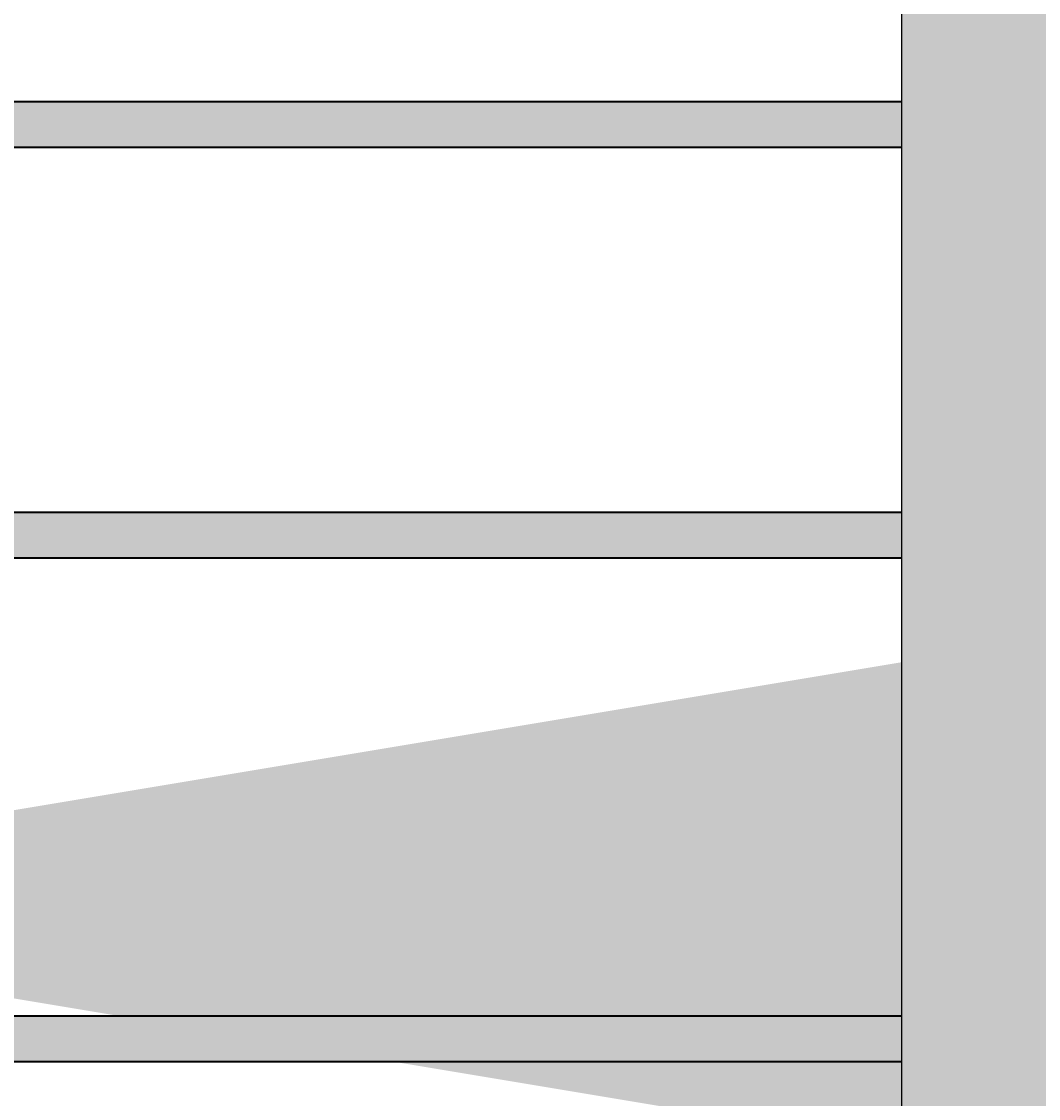
# Model space of a CAD drawing. Units: millimetres. Extents: x -22994 to 29398, y -19990 to 20176.
# Tile 20 of 135: x 77 to 99, y 76 to 99. Entities that reach past the tile are written whole.
import ezdxf

# ---------------------------------------------------------------- set-up
doc = ezdxf.new("R2010")
doc.units = ezdxf.units.MM
doc.header["$MEASUREMENT"] = 0
for name, color, linetype, lineweight in [('M-DIMS', 2, 'Continuous', 18), ('M-EQPM', 7, 'Continuous', 25), ('M-EQPM-PATT', 7, 'Continuous', 18), ('M-PIPE', 7, 'Continuous', 35)]:
    doc.layers.add(name, color=color, linetype=linetype, lineweight=lineweight)
doc.styles.get("Standard").update_dxf_attribs({"font": 'arial.ttf'})
doc.dimstyles.get("Standard").update_dxf_attribs({"dimtxt": 0.18, "dimasz": 10000, "dimexe": 0.18, "dimexo": 0.0625, "dimgap": 0.09, "dimtad": 0, "dimtih": 1, "dimtoh": 1, "dimdec": 0, "dimzin": 0, "dimdsep": 46, "dimtxsty": 'Standard', "dimcen": 0.09, "dimadec": 0, "dimazin": 0, "dimtfac": 1, "dimtdec": 0, "dimtofl": 0, "dimtmove": 0, "dimatfit": 3, "dimfxl": 1, "dimtolj": 1, "dimtzin": 0, "dimlwd": 30, "dimarcsym": 0})

# ---------------------------------------------------------------- blocks, each defined once
blk = doc.blocks.new('*D2')
at = {"layer": 'Defpoints', "color": 0, "transparency": 16777216}
for p in [(6.677, 10.271), (290.852, 10.271), (290.852, -5.079)]:
    blk.add_point(p, dxfattribs=at)
at = {"layer": 'M-DIMS', "color": 0, "lineweight": -2, "transparency": 16777216}
for p, q in [((6.677, 10.209), (6.677, -5.259)), ((290.852, 10.209), (290.852, -5.259))]:
    blk.add_line(p, q, dxfattribs=at)
at = {"layer": 'M-DIMS', "color": 0, "lineweight": 30, "transparency": 16777216}
for p, q in [((-9993.323, -5.079), (-19993.323, -5.079)), ((10290.852, -5.079), (20290.852, -5.079))]:
    blk.add_line(p, q, dxfattribs=at)
at = {"layer": 'M-DIMS', "color": 0, "transparency": 16777216}
for points in [[(-9993.323, 1661.588), (-9993.323, -1671.745), (6.677, -5.079)], [(10290.852, 1661.588), (10290.852, -1671.745), (290.852, -5.079)]]:
    blk.add_solid(points, dxfattribs=at)
at = {"layer": 'M-DIMS', "color": 0, "transparency": 16777216, "insert": (148.765, -5.079), "char_height": 0.18, "attachment_point": 5}
blk.add_mtext('\\A1;284.2', dxfattribs=at)
blk = doc.blocks.new('*D3')
at = {"layer": 'Defpoints', "color": 0, "transparency": 16777216}
for p in [(110.265, 204.165), (110.265, 176.366), (95.833, 127.967)]:
    blk.add_point(p, dxfattribs=at)
at = {"layer": 'M-DIMS', "color": 0, "lineweight": -2, "transparency": 16777216}
for p, q in [((95.833, 128.03), (95.833, 204.345)), ((110.265, 176.429), (110.265, 204.345))]:
    blk.add_line(p, q, dxfattribs=at)
at = {"layer": 'M-DIMS', "color": 0, "lineweight": 30, "transparency": 16777216}
for p, q in [((-9904.167, 204.165), (-19904.167, 204.165)), ((10110.265, 204.165), (20110.265, 204.165))]:
    blk.add_line(p, q, dxfattribs=at)
at = {"layer": 'M-DIMS', "color": 0, "transparency": 16777216}
for points in [[(-9904.167, 1870.832), (-9904.167, -1462.501), (95.833, 204.165)], [(10110.265, 1870.832), (10110.265, -1462.501), (110.265, 204.165)]]:
    blk.add_solid(points, dxfattribs=at)
at = {"layer": 'M-DIMS', "color": 0, "transparency": 16777216, "insert": (103.049, 204.165), "char_height": 0.18, "attachment_point": 5}
blk.add_mtext('\\A1;14.432', dxfattribs=at)
blk = doc.blocks.new('*D4')
at = {"layer": 'Defpoints', "color": 0, "transparency": 16777216}
for p in [(116.265, 204.165), (110.265, 176.366), (116.265, 176.366)]:
    blk.add_point(p, dxfattribs=at)
at = {"layer": 'M-DIMS', "color": 0, "lineweight": -2, "transparency": 16777216}
for p, q in [((110.265, 176.429), (110.265, 204.345)), ((116.265, 176.429), (116.265, 204.345))]:
    blk.add_line(p, q, dxfattribs=at)
at = {"layer": 'M-DIMS', "color": 0, "lineweight": 30, "transparency": 16777216}
for p, q in [((-9889.735, 204.165), (-19889.735, 204.165)), ((10116.265, 204.165), (20116.265, 204.165))]:
    blk.add_line(p, q, dxfattribs=at)
at = {"layer": 'M-DIMS', "color": 0, "transparency": 16777216}
for points in [[(-9889.735, 1870.832), (-9889.735, -1462.501), (110.265, 204.165)], [(10116.265, 1870.832), (10116.265, -1462.501), (116.265, 204.165)]]:
    blk.add_solid(points, dxfattribs=at)
at = {"layer": 'M-DIMS', "color": 0, "transparency": 16777216, "insert": (113.265, 204.165), "char_height": 0.18, "attachment_point": 5}
blk.add_mtext('\\A1;6', dxfattribs=at)
blk = doc.blocks.new('*D5')
at = {"layer": 'Defpoints', "color": 0, "transparency": 16777216}
for p in [(181.265, 204.165), (116.265, 176.366), (181.265, 176.366)]:
    blk.add_point(p, dxfattribs=at)
at = {"layer": 'M-DIMS', "color": 0, "lineweight": -2, "transparency": 16777216}
for p, q in [((116.265, 176.429), (116.265, 204.345)), ((181.265, 176.429), (181.265, 204.345))]:
    blk.add_line(p, q, dxfattribs=at)
at = {"layer": 'M-DIMS', "color": 0, "lineweight": 30, "transparency": 16777216}
for p, q in [((-9883.735, 204.165), (-19883.735, 204.165)), ((10181.265, 204.165), (20181.265, 204.165))]:
    blk.add_line(p, q, dxfattribs=at)
at = {"layer": 'M-DIMS', "color": 0, "transparency": 16777216}
for points in [[(-9883.735, 1870.832), (-9883.735, -1462.501), (116.265, 204.165)], [(10181.265, 1870.832), (10181.265, -1462.501), (181.265, 204.165)]]:
    blk.add_solid(points, dxfattribs=at)
at = {"layer": 'M-DIMS', "color": 0, "transparency": 16777216, "insert": (148.765, 204.165), "char_height": 0.18, "attachment_point": 5}
blk.add_mtext('\\A1;65', dxfattribs=at)
blk = doc.blocks.new('*D6')
at = {"layer": 'Defpoints', "color": 0, "transparency": 16777216}
for p in [(187.265, 204.165), (181.265, 176.366), (187.265, 176.366)]:
    blk.add_point(p, dxfattribs=at)
at = {"layer": 'M-DIMS', "color": 0, "lineweight": -2, "transparency": 16777216}
for p, q in [((181.265, 176.429), (181.265, 204.345)), ((187.265, 176.429), (187.265, 204.345))]:
    blk.add_line(p, q, dxfattribs=at)
at = {"layer": 'M-DIMS', "color": 0, "lineweight": 30, "transparency": 16777216}
for p, q in [((-9818.735, 204.165), (-19818.735, 204.165)), ((10187.265, 204.165), (20187.265, 204.165))]:
    blk.add_line(p, q, dxfattribs=at)
at = {"layer": 'M-DIMS', "color": 0, "transparency": 16777216}
for points in [[(-9818.735, 1870.832), (-9818.735, -1462.501), (181.265, 204.165)], [(10187.265, 1870.832), (10187.265, -1462.501), (187.265, 204.165)]]:
    blk.add_solid(points, dxfattribs=at)
at = {"layer": 'M-DIMS', "color": 0, "transparency": 16777216, "insert": (184.265, 204.165), "char_height": 0.18, "attachment_point": 5}
blk.add_mtext('\\A1;6', dxfattribs=at)
blk = doc.blocks.new('*D7')
at = {"layer": 'Defpoints', "color": 0, "transparency": 16777216}
for p in [(201.697, 204.165), (187.265, 176.366), (201.697, 127.967)]:
    blk.add_point(p, dxfattribs=at)
at = {"layer": 'M-DIMS', "color": 0, "lineweight": -2, "transparency": 16777216}
for p, q in [((187.265, 176.429), (187.265, 204.345)), ((201.697, 128.03), (201.697, 204.345))]:
    blk.add_line(p, q, dxfattribs=at)
at = {"layer": 'M-DIMS', "color": 0, "lineweight": 30, "transparency": 16777216}
for p, q in [((-9812.735, 204.165), (-19812.735, 204.165)), ((10201.697, 204.165), (20201.697, 204.165))]:
    blk.add_line(p, q, dxfattribs=at)
at = {"layer": 'M-DIMS', "color": 0, "transparency": 16777216}
for points in [[(-9812.735, 1870.832), (-9812.735, -1462.501), (187.265, 204.165)], [(10201.697, 1870.832), (10201.697, -1462.501), (201.697, 204.165)]]:
    blk.add_solid(points, dxfattribs=at)
at = {"layer": 'M-DIMS', "color": 0, "transparency": 16777216, "insert": (194.481, 204.165), "char_height": 0.18, "attachment_point": 5}
blk.add_mtext('\\A1;14.432', dxfattribs=at)
blk = doc.blocks.new('*D8')
at = {"layer": 'Defpoints', "color": 0, "transparency": 16777216}
for p in [(227.648, 204.165), (227.648, 146.73), (201.697, 127.967)]:
    blk.add_point(p, dxfattribs=at)
at = {"layer": 'M-DIMS', "color": 0, "lineweight": -2, "transparency": 16777216}
for p, q in [((201.697, 128.03), (201.697, 204.345)), ((227.648, 146.792), (227.648, 204.345))]:
    blk.add_line(p, q, dxfattribs=at)
at = {"layer": 'M-DIMS', "color": 0, "lineweight": 30, "transparency": 16777216}
for p, q in [((-9798.303, 204.165), (-19798.303, 204.165)), ((10227.648, 204.165), (20227.648, 204.165))]:
    blk.add_line(p, q, dxfattribs=at)
at = {"layer": 'M-DIMS', "color": 0, "transparency": 16777216}
for points in [[(-9798.303, 1870.832), (-9798.303, -1462.501), (201.697, 204.165)], [(10227.648, 1870.832), (10227.648, -1462.501), (227.648, 204.165)]]:
    blk.add_solid(points, dxfattribs=at)
at = {"layer": 'M-DIMS', "color": 0, "transparency": 16777216, "insert": (214.673, 204.165), "char_height": 0.18, "attachment_point": 5}
blk.add_mtext('\\A1;25.95', dxfattribs=at)
blk = doc.blocks.new('*D9')
at = {"layer": 'Defpoints', "color": 0, "transparency": 16777216}
for p in [(187.265, 176.366), (306.202, 176.366), (290.852, 10.271)]:
    blk.add_point(p, dxfattribs=at)
at = {"layer": 'M-DIMS', "color": 0, "lineweight": 30, "transparency": 16777216}
for p, q in [((306.202, 10176.366), (306.202, 20176.366)), ((306.202, -9989.729), (306.202, -19989.729))]:
    blk.add_line(p, q, dxfattribs=at)
at = {"layer": 'M-DIMS', "color": 0, "lineweight": -2, "transparency": 16777216}
for p, q in [((187.327, 176.366), (306.382, 176.366)), ((290.915, 10.271), (306.382, 10.271))]:
    blk.add_line(p, q, dxfattribs=at)
at = {"layer": 'M-DIMS', "color": 0, "transparency": 16777216}
for points in [[(-1360.465, 10176.366), (1972.869, 10176.366), (306.202, 176.366)], [(-1360.465, -9989.729), (1972.869, -9989.729), (306.202, 10.271)]]:
    blk.add_solid(points, dxfattribs=at)
at = {"layer": 'M-DIMS', "color": 0, "transparency": 16777216, "insert": (306.202, 93.319), "char_height": 0.18, "attachment_point": 5}
blk.add_mtext('\\A1;166.1', dxfattribs=at)
blk = doc.blocks.new('*D10')
at = {"layer": 'Defpoints', "color": 0, "transparency": 16777216}
for p in [(125.65, 136.071), (133.346, 136.071), (133.346, -5.079)]:
    blk.add_point(p, dxfattribs=at)
at = {"layer": 'M-DIMS', "color": 0, "lineweight": -2, "transparency": 16777216}
for p, q in [((125.65, 136.009), (125.65, -5.259)), ((133.346, 136.009), (133.346, -5.259))]:
    blk.add_line(p, q, dxfattribs=at)
at = {"layer": 'M-DIMS', "color": 0, "lineweight": 30, "transparency": 16777216}
for p, q in [((-9874.35, -5.079), (-19874.35, -5.079)), ((10133.346, -5.079), (20133.346, -5.079))]:
    blk.add_line(p, q, dxfattribs=at)
at = {"layer": 'M-DIMS', "color": 0, "transparency": 16777216}
for points in [[(-9874.35, 1661.588), (-9874.35, -1671.745), (125.65, -5.079)], [(10133.346, 1661.588), (10133.346, -1671.745), (133.346, -5.079)]]:
    blk.add_solid(points, dxfattribs=at)
at = {"layer": 'M-DIMS', "color": 0, "transparency": 16777216, "insert": (129.498, -5.079), "char_height": 0.18, "attachment_point": 5}
blk.add_mtext('\\A1;7.696', dxfattribs=at)
blk = doc.blocks.new('*D11')
at = {"layer": 'Defpoints', "color": 0, "transparency": 16777216}
for p in [(133.346, 136.071), (135.65, 136.071), (135.65, -5.079)]:
    blk.add_point(p, dxfattribs=at)
at = {"layer": 'M-DIMS', "color": 0, "lineweight": -2, "transparency": 16777216}
for p, q in [((133.346, 136.009), (133.346, -5.259)), ((135.65, 136.009), (135.65, -5.259))]:
    blk.add_line(p, q, dxfattribs=at)
at = {"layer": 'M-DIMS', "color": 0, "lineweight": 30, "transparency": 16777216}
for p, q in [((-9866.654, -5.079), (-19866.654, -5.079)), ((10135.65, -5.079), (20135.65, -5.079))]:
    blk.add_line(p, q, dxfattribs=at)
at = {"layer": 'M-DIMS', "color": 0, "transparency": 16777216}
for points in [[(-9866.654, 1661.588), (-9866.654, -1671.745), (133.346, -5.079)], [(10135.65, 1661.588), (10135.65, -1671.745), (135.65, -5.079)]]:
    blk.add_solid(points, dxfattribs=at)
at = {"layer": 'M-DIMS', "color": 0, "transparency": 16777216, "insert": (134.498, -5.079), "char_height": 0.18, "attachment_point": 5}
blk.add_mtext('\\A1;2.304', dxfattribs=at)
blk = doc.blocks.new('*D12')
at = {"layer": 'Defpoints', "color": 0, "transparency": 16777216}
for p in [(135.65, 136.071), (145.65, 136.071), (145.65, -5.079)]:
    blk.add_point(p, dxfattribs=at)
at = {"layer": 'M-DIMS', "color": 0, "lineweight": -2, "transparency": 16777216}
for p, q in [((135.65, 136.009), (135.65, -5.259)), ((145.65, 136.009), (145.65, -5.259))]:
    blk.add_line(p, q, dxfattribs=at)
at = {"layer": 'M-DIMS', "color": 0, "lineweight": 30, "transparency": 16777216}
for p, q in [((-9864.35, -5.079), (-19864.35, -5.079)), ((10145.65, -5.079), (20145.65, -5.079))]:
    blk.add_line(p, q, dxfattribs=at)
at = {"layer": 'M-DIMS', "color": 0, "transparency": 16777216}
for points in [[(-9864.35, 1661.588), (-9864.35, -1671.745), (135.65, -5.079)], [(10145.65, 1661.588), (10145.65, -1671.745), (145.65, -5.079)]]:
    blk.add_solid(points, dxfattribs=at)
at = {"layer": 'M-DIMS', "color": 0, "transparency": 16777216, "insert": (140.65, -5.079), "char_height": 0.18, "attachment_point": 5}
blk.add_mtext('\\A1;10', dxfattribs=at)
blk = doc.blocks.new('*D13')
at = {"layer": 'Defpoints', "color": 0, "transparency": 16777216}
for p in [(145.65, 136.071), (155.65, 136.071), (155.65, -5.079)]:
    blk.add_point(p, dxfattribs=at)
at = {"layer": 'M-DIMS', "color": 0, "lineweight": -2, "transparency": 16777216}
for p, q in [((145.65, 136.009), (145.65, -5.259)), ((155.65, 136.009), (155.65, -5.259))]:
    blk.add_line(p, q, dxfattribs=at)
at = {"layer": 'M-DIMS', "color": 0, "lineweight": 30, "transparency": 16777216}
for p, q in [((-9854.35, -5.079), (-19854.35, -5.079)), ((10155.65, -5.079), (20155.65, -5.079))]:
    blk.add_line(p, q, dxfattribs=at)
at = {"layer": 'M-DIMS', "color": 0, "transparency": 16777216}
for points in [[(-9854.35, 1661.588), (-9854.35, -1671.745), (145.65, -5.079)], [(10155.65, 1661.588), (10155.65, -1671.745), (155.65, -5.079)]]:
    blk.add_solid(points, dxfattribs=at)
at = {"layer": 'M-DIMS', "color": 0, "transparency": 16777216, "insert": (150.65, -5.079), "char_height": 0.18, "attachment_point": 5}
blk.add_mtext('\\A1;10', dxfattribs=at)
blk = doc.blocks.new('*D14')
at = {"layer": 'Defpoints', "color": 0, "transparency": 16777216}
for p in [(155.65, 136.071), (165.65, 136.071), (165.65, -5.079)]:
    blk.add_point(p, dxfattribs=at)
at = {"layer": 'M-DIMS', "color": 0, "lineweight": -2, "transparency": 16777216}
for p, q in [((155.65, 136.009), (155.65, -5.259)), ((165.65, 136.009), (165.65, -5.259))]:
    blk.add_line(p, q, dxfattribs=at)
at = {"layer": 'M-DIMS', "color": 0, "lineweight": 30, "transparency": 16777216}
for p, q in [((-9844.35, -5.079), (-19844.35, -5.079)), ((10165.65, -5.079), (20165.65, -5.079))]:
    blk.add_line(p, q, dxfattribs=at)
at = {"layer": 'M-DIMS', "color": 0, "transparency": 16777216}
for points in [[(-9844.35, 1661.588), (-9844.35, -1671.745), (155.65, -5.079)], [(10165.65, 1661.588), (10165.65, -1671.745), (165.65, -5.079)]]:
    blk.add_solid(points, dxfattribs=at)
at = {"layer": 'M-DIMS', "color": 0, "transparency": 16777216, "insert": (160.65, -5.079), "char_height": 0.18, "attachment_point": 5}
blk.add_mtext('\\A1;10', dxfattribs=at)
blk = doc.blocks.new('*D15')
at = {"layer": 'Defpoints', "color": 0, "transparency": 16777216}
for p in [(173.346, 154.788), (173.346, 136.071), (306.202, 136.071)]:
    blk.add_point(p, dxfattribs=at)
at = {"layer": 'M-DIMS', "color": 0, "lineweight": 30, "transparency": 16777216}
for p, q in [((306.202, 10154.788), (306.202, 20154.788)), ((306.202, -9863.929), (306.202, -19863.929))]:
    blk.add_line(p, q, dxfattribs=at)
at = {"layer": 'M-DIMS', "color": 0, "lineweight": -2, "transparency": 16777216}
for p, q in [((173.408, 154.788), (306.382, 154.788)), ((173.408, 136.071), (306.382, 136.071))]:
    blk.add_line(p, q, dxfattribs=at)
at = {"layer": 'M-DIMS', "color": 0, "transparency": 16777216}
for points in [[(-1360.465, 10154.788), (1972.869, 10154.788), (306.202, 154.788)], [(-1360.465, -9863.929), (1972.869, -9863.929), (306.202, 136.071)]]:
    blk.add_solid(points, dxfattribs=at)
at = {"layer": 'M-DIMS', "color": 0, "transparency": 16777216, "insert": (306.202, 145.43), "char_height": 0.18, "attachment_point": 5}
blk.add_mtext('\\A1;18.717', dxfattribs=at)
blk = doc.blocks.new('*D16')
at = {"layer": 'Defpoints', "color": 0, "transparency": 16777216}
for p in [(120.17, 204.165), (110.466, 48.035), (120.17, 48.035)]:
    blk.add_point(p, dxfattribs=at)
at = {"layer": 'M-DIMS', "color": 0, "lineweight": -2, "transparency": 16777216}
for p, q in [((110.466, 48.097), (110.466, 204.345)), ((120.17, 48.097), (120.17, 204.345))]:
    blk.add_line(p, q, dxfattribs=at)
at = {"layer": 'M-DIMS', "color": 0, "lineweight": 30, "transparency": 16777216}
for p, q in [((-9889.534, 204.165), (-19889.534, 204.165)), ((10120.17, 204.165), (20120.17, 204.165))]:
    blk.add_line(p, q, dxfattribs=at)
at = {"layer": 'M-DIMS', "color": 0, "transparency": 16777216}
for points in [[(-9889.534, 1870.832), (-9889.534, -1462.501), (110.466, 204.165)], [(10120.17, 1870.832), (10120.17, -1462.501), (120.17, 204.165)]]:
    blk.add_solid(points, dxfattribs=at)
at = {"layer": 'M-DIMS', "color": 0, "transparency": 16777216, "insert": (115.318, 204.165), "char_height": 0.18, "attachment_point": 5}
blk.add_mtext('\\A1;9.704', dxfattribs=at)
blk = doc.blocks.new('*D17')
at = {"layer": 'Defpoints', "color": 0, "transparency": 16777216}
for p in [(126.17, 204.165), (120.17, 48.035), (126.17, 48.035)]:
    blk.add_point(p, dxfattribs=at)
at = {"layer": 'M-DIMS', "color": 0, "lineweight": -2, "transparency": 16777216}
for p, q in [((120.17, 48.097), (120.17, 204.345)), ((126.17, 48.097), (126.17, 204.345))]:
    blk.add_line(p, q, dxfattribs=at)
at = {"layer": 'M-DIMS', "color": 0, "lineweight": 30, "transparency": 16777216}
for p, q in [((-9879.83, 204.165), (-19879.83, 204.165)), ((10126.17, 204.165), (20126.17, 204.165))]:
    blk.add_line(p, q, dxfattribs=at)
at = {"layer": 'M-DIMS', "color": 0, "transparency": 16777216}
for points in [[(-9879.83, 1870.832), (-9879.83, -1462.501), (120.17, 204.165)], [(10126.17, 1870.832), (10126.17, -1462.501), (126.17, 204.165)]]:
    blk.add_solid(points, dxfattribs=at)
at = {"layer": 'M-DIMS', "color": 0, "transparency": 16777216, "insert": (123.17, 204.165), "char_height": 0.18, "attachment_point": 5}
blk.add_mtext('\\A1;6', dxfattribs=at)
blk = doc.blocks.new('*D18')
at = {"layer": 'Defpoints', "color": 0, "transparency": 16777216}
for p in [(132.17, 204.165), (126.17, 48.035), (132.17, 48.035)]:
    blk.add_point(p, dxfattribs=at)
at = {"layer": 'M-DIMS', "color": 0, "lineweight": -2, "transparency": 16777216}
for p, q in [((126.17, 48.097), (126.17, 204.345)), ((132.17, 48.097), (132.17, 204.345))]:
    blk.add_line(p, q, dxfattribs=at)
at = {"layer": 'M-DIMS', "color": 0, "lineweight": 30, "transparency": 16777216}
for p, q in [((-9873.83, 204.165), (-19873.83, 204.165)), ((10132.17, 204.165), (20132.17, 204.165))]:
    blk.add_line(p, q, dxfattribs=at)
at = {"layer": 'M-DIMS', "color": 0, "transparency": 16777216}
for points in [[(-9873.83, 1870.832), (-9873.83, -1462.501), (126.17, 204.165)], [(10132.17, 1870.832), (10132.17, -1462.501), (132.17, 204.165)]]:
    blk.add_solid(points, dxfattribs=at)
at = {"layer": 'M-DIMS', "color": 0, "transparency": 16777216, "insert": (129.17, 204.165), "char_height": 0.18, "attachment_point": 5}
blk.add_mtext('\\A1;6', dxfattribs=at)
blk = doc.blocks.new('*D19')
at = {"layer": 'Defpoints', "color": 0, "transparency": 16777216}
for p in [(138.17, 204.165), (132.17, 48.035), (138.17, 48.035)]:
    blk.add_point(p, dxfattribs=at)
at = {"layer": 'M-DIMS', "color": 0, "lineweight": -2, "transparency": 16777216}
for p, q in [((132.17, 48.097), (132.17, 204.345)), ((138.17, 48.097), (138.17, 204.345))]:
    blk.add_line(p, q, dxfattribs=at)
at = {"layer": 'M-DIMS', "color": 0, "lineweight": 30, "transparency": 16777216}
for p, q in [((-9867.83, 204.165), (-19867.83, 204.165)), ((10138.17, 204.165), (20138.17, 204.165))]:
    blk.add_line(p, q, dxfattribs=at)
at = {"layer": 'M-DIMS', "color": 0, "transparency": 16777216}
for points in [[(-9867.83, 1870.832), (-9867.83, -1462.501), (132.17, 204.165)], [(10138.17, 1870.832), (10138.17, -1462.501), (138.17, 204.165)]]:
    blk.add_solid(points, dxfattribs=at)
at = {"layer": 'M-DIMS', "color": 0, "transparency": 16777216, "insert": (135.17, 204.165), "char_height": 0.18, "attachment_point": 5}
blk.add_mtext('\\A1;6', dxfattribs=at)
blk = doc.blocks.new('*D20')
at = {"layer": 'Defpoints', "color": 0, "transparency": 16777216}
for p in [(144.17, 204.165), (138.17, 48.035), (144.17, 48.035)]:
    blk.add_point(p, dxfattribs=at)
at = {"layer": 'M-DIMS', "color": 0, "lineweight": -2, "transparency": 16777216}
for p, q in [((138.17, 48.097), (138.17, 204.345)), ((144.17, 48.097), (144.17, 204.345))]:
    blk.add_line(p, q, dxfattribs=at)
at = {"layer": 'M-DIMS', "color": 0, "lineweight": 30, "transparency": 16777216}
for p, q in [((-9861.83, 204.165), (-19861.83, 204.165)), ((10144.17, 204.165), (20144.17, 204.165))]:
    blk.add_line(p, q, dxfattribs=at)
at = {"layer": 'M-DIMS', "color": 0, "transparency": 16777216}
for points in [[(-9861.83, 1870.832), (-9861.83, -1462.501), (138.17, 204.165)], [(10144.17, 1870.832), (10144.17, -1462.501), (144.17, 204.165)]]:
    blk.add_solid(points, dxfattribs=at)
at = {"layer": 'M-DIMS', "color": 0, "transparency": 16777216, "insert": (141.17, 204.165), "char_height": 0.18, "attachment_point": 5}
blk.add_mtext('\\A1;6', dxfattribs=at)
blk = doc.blocks.new('*D21')
at = {"layer": 'Defpoints', "color": 0, "transparency": 16777216}
for p in [(149.116, 204.165), (144.17, 48.035), (149.116, 48.035)]:
    blk.add_point(p, dxfattribs=at)
at = {"layer": 'M-DIMS', "color": 0, "lineweight": -2, "transparency": 16777216}
for p, q in [((144.17, 48.097), (144.17, 204.345)), ((149.116, 48.097), (149.116, 204.345))]:
    blk.add_line(p, q, dxfattribs=at)
at = {"layer": 'M-DIMS', "color": 0, "lineweight": 30, "transparency": 16777216}
for p, q in [((-9855.83, 204.165), (-19855.83, 204.165)), ((10149.116, 204.165), (20149.116, 204.165))]:
    blk.add_line(p, q, dxfattribs=at)
at = {"layer": 'M-DIMS', "color": 0, "transparency": 16777216}
for points in [[(-9855.83, 1870.832), (-9855.83, -1462.501), (144.17, 204.165)], [(10149.116, 1870.832), (10149.116, -1462.501), (149.116, 204.165)]]:
    blk.add_solid(points, dxfattribs=at)
at = {"layer": 'M-DIMS', "color": 0, "transparency": 16777216, "insert": (146.643, 204.165), "char_height": 0.18, "attachment_point": 5}
blk.add_mtext('\\A1;4.945', dxfattribs=at)
blk = doc.blocks.new('*D22')
at = {"layer": 'Defpoints', "color": 0, "transparency": 16777216}
for p in [(149.116, 30.99), (155.116, 30.99), (155.116, -5.079)]:
    blk.add_point(p, dxfattribs=at)
at = {"layer": 'M-DIMS', "color": 0, "lineweight": -2, "transparency": 16777216}
for p, q in [((149.116, 30.927), (149.116, -5.259)), ((155.116, 30.927), (155.116, -5.259))]:
    blk.add_line(p, q, dxfattribs=at)
at = {"layer": 'M-DIMS', "color": 0, "lineweight": 30, "transparency": 16777216}
for p, q in [((-9850.884, -5.079), (-19850.884, -5.079)), ((10155.116, -5.079), (20155.116, -5.079))]:
    blk.add_line(p, q, dxfattribs=at)
at = {"layer": 'M-DIMS', "color": 0, "transparency": 16777216}
for points in [[(-9850.884, 1661.588), (-9850.884, -1671.745), (149.116, -5.079)], [(10155.116, 1661.588), (10155.116, -1671.745), (155.116, -5.079)]]:
    blk.add_solid(points, dxfattribs=at)
at = {"layer": 'M-DIMS', "color": 0, "transparency": 16777216, "insert": (152.116, -5.079), "char_height": 0.18, "attachment_point": 5}
blk.add_mtext('\\A1;6', dxfattribs=at)
blk = doc.blocks.new('*D23')
at = {"layer": 'Defpoints', "color": 0, "transparency": 16777216}
for p in [(155.116, 30.99), (161.116, 30.99), (161.116, -5.079)]:
    blk.add_point(p, dxfattribs=at)
at = {"layer": 'M-DIMS', "color": 0, "lineweight": -2, "transparency": 16777216}
for p, q in [((155.116, 30.927), (155.116, -5.259)), ((161.116, 30.927), (161.116, -5.259))]:
    blk.add_line(p, q, dxfattribs=at)
at = {"layer": 'M-DIMS', "color": 0, "lineweight": 30, "transparency": 16777216}
for p, q in [((-9844.884, -5.079), (-19844.884, -5.079)), ((10161.116, -5.079), (20161.116, -5.079))]:
    blk.add_line(p, q, dxfattribs=at)
at = {"layer": 'M-DIMS', "color": 0, "transparency": 16777216}
for points in [[(-9844.884, 1661.588), (-9844.884, -1671.745), (155.116, -5.079)], [(10161.116, 1661.588), (10161.116, -1671.745), (161.116, -5.079)]]:
    blk.add_solid(points, dxfattribs=at)
at = {"layer": 'M-DIMS', "color": 0, "transparency": 16777216, "insert": (158.116, -5.079), "char_height": 0.18, "attachment_point": 5}
blk.add_mtext('\\A1;6', dxfattribs=at)
blk = doc.blocks.new('*D24')
at = {"layer": 'Defpoints', "color": 0, "transparency": 16777216}
for p in [(161.116, 30.99), (166.439, 30.99), (166.439, -5.079)]:
    blk.add_point(p, dxfattribs=at)
at = {"layer": 'M-DIMS', "color": 0, "lineweight": -2, "transparency": 16777216}
for p, q in [((161.116, 30.927), (161.116, -5.259)), ((166.439, 30.927), (166.439, -5.259))]:
    blk.add_line(p, q, dxfattribs=at)
at = {"layer": 'M-DIMS', "color": 0, "lineweight": 30, "transparency": 16777216}
for p, q in [((-9838.884, -5.079), (-19838.884, -5.079)), ((10166.439, -5.079), (20166.439, -5.079))]:
    blk.add_line(p, q, dxfattribs=at)
at = {"layer": 'M-DIMS', "color": 0, "transparency": 16777216}
for points in [[(-9838.884, 1661.588), (-9838.884, -1671.745), (161.116, -5.079)], [(10166.439, 1661.588), (10166.439, -1671.745), (166.439, -5.079)]]:
    blk.add_solid(points, dxfattribs=at)
at = {"layer": 'M-DIMS', "color": 0, "transparency": 16777216, "insert": (163.777, -5.079), "char_height": 0.18, "attachment_point": 5}
blk.add_mtext('\\A1;5.323', dxfattribs=at)
blk = doc.blocks.new('*D25')
at = {"layer": 'Defpoints', "color": 0, "transparency": 16777216}
for p in [(166.439, 30.99), (172.439, 30.99), (172.439, -5.079)]:
    blk.add_point(p, dxfattribs=at)
at = {"layer": 'M-DIMS', "color": 0, "lineweight": -2, "transparency": 16777216}
for p, q in [((166.439, 30.927), (166.439, -5.259)), ((172.439, 30.927), (172.439, -5.259))]:
    blk.add_line(p, q, dxfattribs=at)
at = {"layer": 'M-DIMS', "color": 0, "lineweight": 30, "transparency": 16777216}
for p, q in [((-9833.561, -5.079), (-19833.561, -5.079)), ((10172.439, -5.079), (20172.439, -5.079))]:
    blk.add_line(p, q, dxfattribs=at)
at = {"layer": 'M-DIMS', "color": 0, "transparency": 16777216}
for points in [[(-9833.561, 1661.588), (-9833.561, -1671.745), (166.439, -5.079)], [(10172.439, 1661.588), (10172.439, -1671.745), (172.439, -5.079)]]:
    blk.add_solid(points, dxfattribs=at)
at = {"layer": 'M-DIMS', "color": 0, "transparency": 16777216, "insert": (169.439, -5.079), "char_height": 0.18, "attachment_point": 5}
blk.add_mtext('\\A1;6', dxfattribs=at)
blk = doc.blocks.new('*D26')
at = {"layer": 'Defpoints', "color": 0, "transparency": 16777216}
for p in [(172.439, 30.99), (178.439, 30.99), (178.439, -5.079)]:
    blk.add_point(p, dxfattribs=at)
at = {"layer": 'M-DIMS', "color": 0, "lineweight": -2, "transparency": 16777216}
for p, q in [((172.439, 30.927), (172.439, -5.259)), ((178.439, 30.927), (178.439, -5.259))]:
    blk.add_line(p, q, dxfattribs=at)
at = {"layer": 'M-DIMS', "color": 0, "lineweight": 30, "transparency": 16777216}
for p, q in [((-9827.561, -5.079), (-19827.561, -5.079)), ((10178.439, -5.079), (20178.439, -5.079))]:
    blk.add_line(p, q, dxfattribs=at)
at = {"layer": 'M-DIMS', "color": 0, "transparency": 16777216}
for points in [[(-9827.561, 1661.588), (-9827.561, -1671.745), (172.439, -5.079)], [(10178.439, 1661.588), (10178.439, -1671.745), (178.439, -5.079)]]:
    blk.add_solid(points, dxfattribs=at)
at = {"layer": 'M-DIMS', "color": 0, "transparency": 16777216, "insert": (175.439, -5.079), "char_height": 0.18, "attachment_point": 5}
blk.add_mtext('\\A1;6', dxfattribs=at)
blk = doc.blocks.new('*D27')
at = {"layer": 'Defpoints', "color": 0, "transparency": 16777216}
for p in [(178.439, 30.99), (188.117, 30.99), (188.117, -5.079)]:
    blk.add_point(p, dxfattribs=at)
at = {"layer": 'M-DIMS', "color": 0, "lineweight": -2, "transparency": 16777216}
for p, q in [((178.439, 30.927), (178.439, -5.259)), ((188.117, 30.927), (188.117, -5.259))]:
    blk.add_line(p, q, dxfattribs=at)
at = {"layer": 'M-DIMS', "color": 0, "lineweight": 30, "transparency": 16777216}
for p, q in [((-9821.561, -5.079), (-19821.561, -5.079)), ((10188.117, -5.079), (20188.117, -5.079))]:
    blk.add_line(p, q, dxfattribs=at)
at = {"layer": 'M-DIMS', "color": 0, "transparency": 16777216}
for points in [[(-9821.561, 1661.588), (-9821.561, -1671.745), (178.439, -5.079)], [(10188.117, 1661.588), (10188.117, -1671.745), (188.117, -5.079)]]:
    blk.add_solid(points, dxfattribs=at)
at = {"layer": 'M-DIMS', "color": 0, "transparency": 16777216, "insert": (183.278, -5.079), "char_height": 0.18, "attachment_point": 5}
blk.add_mtext('\\A1;9.679', dxfattribs=at)
blk = doc.blocks.new('*D28')
at = {"layer": 'Defpoints', "color": 0, "transparency": 16777216}
for p in [(188.117, 48.035), (306.202, 48.035), (188.117, 30.99)]:
    blk.add_point(p, dxfattribs=at)
at = {"layer": 'M-DIMS', "color": 0, "lineweight": 30, "transparency": 16777216}
for p, q in [((306.202, 10048.035), (306.202, 20048.035)), ((306.202, -9969.01), (306.202, -19969.01))]:
    blk.add_line(p, q, dxfattribs=at)
at = {"layer": 'M-DIMS', "color": 0, "lineweight": -2, "transparency": 16777216}
for p, q in [((188.18, 48.035), (306.382, 48.035)), ((188.18, 30.99), (306.382, 30.99))]:
    blk.add_line(p, q, dxfattribs=at)
at = {"layer": 'M-DIMS', "color": 0, "transparency": 16777216}
for points in [[(-1360.465, 10048.035), (1972.869, 10048.035), (306.202, 48.035)], [(-1360.465, -9969.01), (1972.869, -9969.01), (306.202, 30.99)]]:
    blk.add_solid(points, dxfattribs=at)
at = {"layer": 'M-DIMS', "color": 0, "transparency": 16777216, "insert": (306.202, 39.512), "char_height": 0.18, "attachment_point": 5}
blk.add_mtext('\\A1;17.045', dxfattribs=at)
blk = doc.blocks.new('*D29')
at = {"layer": 'Defpoints', "color": 0, "transparency": 16777216}
for p in [(36.801, 80.045), (64.03, 80.045)]:
    blk.add_point(p, dxfattribs=at)
at = {"layer": 'M-DIMS', "color": 0, "lineweight": -2, "transparency": 16777216}
for p, q in [((50.325, 80.045), (50.505, 80.045)), ((50.415, 79.955), (50.415, 80.135))]:
    blk.add_line(p, q, dxfattribs=at)
at = {"layer": 'M-DIMS', "color": 0, "lineweight": 30, "transparency": 16777216}
blk.add_line((20064.03, 80.03), (10064.03, 80.038), dxfattribs=at)
at = {"layer": 'M-DIMS', "color": 0, "transparency": 16777216}
blk.add_solid([(10064.031, 1746.704), (10064.028, -1586.629), (64.03, 80.045)], dxfattribs=at)
at = {"layer": 'M-DIMS', "color": 0, "transparency": 16777216, "insert": (20064.521, 80.03), "char_height": 0.18, "attachment_point": 5}
blk.add_mtext('\\A1;∅27.23', dxfattribs=at)
blk = doc.blocks.new('*D36')
at = {"layer": 'Defpoints', "color": 0, "transparency": 16777216}
for p in [(46.39, 31.303), (46.387, 26.593)]:
    blk.add_point(p, dxfattribs=at)
at = {"layer": 'M-DIMS', "color": 0, "lineweight": 30, "transparency": 16777216}
for p, q in [((57.15, 20031.301), (51.77, 10031.302)), ((10057.15, 20031.301), (57.15, 20031.301))]:
    blk.add_line(p, q, dxfattribs=at)
at = {"layer": 'M-DIMS', "color": 0, "lineweight": -2, "transparency": 16777216}
for p, q in [((46.389, 28.858), (46.389, 29.038)), ((46.299, 28.948), (46.479, 28.948))]:
    blk.add_line(p, q, dxfattribs=at)
at = {"layer": 'M-DIMS', "color": 0, "transparency": 16777216}
blk.add_solid([(-1614.896, 10032.199), (1718.436, 10030.405), (46.39, 31.303)], dxfattribs=at)
at = {"layer": 'M-DIMS', "color": 0, "transparency": 16777216, "insert": (10057.554, 20031.301), "char_height": 0.18, "attachment_point": 5}
blk.add_mtext('\\A1;∅4.71', dxfattribs=at)
blk = doc.blocks.new('*D37')
at = {"layer": 'Defpoints', "color": 0, "transparency": 16777216}
for p in [(54.834, 118.615), (59.494, 118.614)]:
    blk.add_point(p, dxfattribs=at)
at = {"layer": 'M-DIMS', "color": 0, "lineweight": -2, "transparency": 16777216}
for p, q in [((57.164, 118.524), (57.164, 118.704)), ((57.074, 118.614), (57.254, 118.614))]:
    blk.add_line(p, q, dxfattribs=at)
at = {"layer": 'M-DIMS', "color": 0, "lineweight": 30, "transparency": 16777216}
blk.add_line((20059.493, 116.253), (10059.494, 117.434), dxfattribs=at)
at = {"layer": 'M-DIMS', "color": 0, "transparency": 16777216}
blk.add_solid([(10059.69, 1784.1), (10059.297, -1549.233), (59.494, 118.614)], dxfattribs=at)
at = {"layer": 'M-DIMS', "color": 0, "transparency": 16777216, "insert": (20059.985, 116.253), "char_height": 0.18, "attachment_point": 5}
blk.add_mtext('\\A1;∅4.659', dxfattribs=at)

msp = doc.modelspace()

# ---------------------------------------------------------------- hatches: boundary and pattern name
at = {"layer": 'M-EQPM-PATT'}
h = msp.add_hatch(color=256, dxfattribs=at)
h.set_gradient(color1=(205, 32, 39), color2=(205, 32, 39), tint=1)
h.paths.add_polyline_path([(116.2647, 150.3662), (116.2647, 170.3662), (116.2647, 176.3662), (110.2647, 176.3662), (110.2647, 152.0276), (95.8327, 127.967), (95.8327, 16.6063), (201.6967, 16.6063), (201.6967, 127.967), (187.2647, 152.0276), (187.2647, 176.3662), (181.2647, 176.3662), (181.2647, 170.3662), (181.2647, 150.3662), (195.6967, 126.3055), (195.6967, 22.6063), (101.8327, 22.6063), (101.8327, 126.3055)])
h.paths.add_polyline_path([(185.2208, 88.6347), (101.8327, 88.6347), (101.8327, 87.6347), (182.8066, 87.6347), (178.7313, 83.5594), (195.6967, 83.5594), (195.6967, 84.5594), (181.1455, 84.5594)], flags=17)
h.paths.add_polyline_path([(95.8327, 88.6347), (60.9779, 88.6347, -0.0228552), (61.7178, 87.6347), (95.8327, 87.6347)])
h.paths.add_polyline_path([(215.6212, 86.5189), (215.6212, 80.5999), (220.5095, 83.5594)])
h.paths.add_polyline_path([(215.6212, 84.5594), (201.6967, 84.5594), (201.6967, 83.5594), (215.6212, 83.5594)])
h.paths.add_polyline_path([(225.3978, 86.5189), (220.5095, 83.5594), (225.3978, 80.5999)])
h.paths.add_polyline_path([(231.6256, 84.5594), (225.3978, 84.5594), (225.3978, 83.5594), (231.6256, 83.5594)])
h = msp.add_hatch(color=256, dxfattribs=at)
h.set_gradient(color1=(34, 52, 110), color2=(41, 49, 137), tint=1, name='CYLINDER')
h.paths.add_polyline_path([(101.8327, 123.6277), (101.8327, 122.6277), (176.8123, 122.6277, -0.4142136), (178.3123, 121.1277), (178.3123, 119.1277, -0.4142136), (176.8123, 117.6277), (129.8123, 117.6277, 0.4142136), (128.3123, 116.1277), (128.3123, 114.1277, 0.4142136), (129.8123, 112.6277), (176.8123, 112.6277, -0.4142136), (178.3123, 111.1277), (178.3123, 109.1277, -0.4142136), (176.8123, 107.6277), (129.8123, 107.6277, 0.4142136), (128.3123, 106.1277), (128.3123, 104.1277, 0.4142136), (129.8123, 102.6277), (176.8123, 102.6277, -0.4142136), (178.3123, 101.1277), (178.3123, 99.1277, -0.4142136), (176.8123, 97.6277), (101.8327, 97.6277), (101.8327, 96.6277), (176.8123, 96.6277, 0.4142136), (179.3123, 99.1277), (179.3123, 101.1277, 0.4142136), (176.8123, 103.6277), (129.8123, 103.6277, -0.4142136), (129.3123, 104.1277), (129.3123, 106.1277, -0.4142136), (129.8123, 106.6277), (176.8123, 106.6277, 0.4142136), (179.3123, 109.1277), (179.3123, 111.1277, 0.4142136), (176.8123, 113.6277), (129.8123, 113.6277, -0.4142136), (129.3123, 114.1277), (129.3123, 116.1277, -0.4142136), (129.8123, 116.6277), (176.8123, 116.6277, 0.4142136), (179.3123, 119.1277), (179.3123, 121.1277, 0.4142136), (176.8123, 123.6277)])
h.paths.add_polyline_path([(75.6657, 123.6277), (75.6657, 122.6277), (95.8327, 122.6277), (95.8327, 123.6277)])
h.paths.add_polyline_path([(51.0853, 122.6277, -0.0439182), (51.8797, 123.6277), (38.9157, 123.6277), (38.9157, 122.6277)])
h.paths.add_polyline_path([(95.8327, 96.6277), (95.8327, 97.6277), (22.2694, 97.6277, 0.4142136), (20.7694, 96.1277), (20.7694, 89.8712, 0.4142136), (22.2694, 88.3712), (39.6435, 88.3712, -0.024152), (40.4967, 89.3712), (23.2694, 89.3712, -0.4142136), (21.7694, 90.8712), (21.7694, 95.1277, -0.4142136), (23.2694, 96.6277)])
h.paths.add_polyline_path([(137.7248, 106.4435), (168.6853, 106.4435), (168.6853, 114.6864), (137.7248, 114.6864)], flags=25)
h = msp.add_hatch(color=256, dxfattribs=at)
h.set_gradient(color1=(19, 155, 72), color2=(88, 186, 72), tint=1, name='CYLINDER')
h.paths.add_polyline_path([(63.8069, 77.5922, -0.0188178), (63.5845, 76.5922), (95.8327, 76.5922), (95.8327, 77.5922)])

# ---------------------------------------------------------------- linework, layer by layer
at = {"layer": 'M-EQPM'}
msp.add_lwpolyline([(110.2647, 176.3662), (110.2647, 152.0276), (95.8327, 127.967), (95.8327, 16.6063), (201.6967, 16.6063), (201.6967, 127.967), (187.2647, 152.0276), (187.2647, 176.3662)], close=True, dxfattribs=at)
at = {"layer": 'M-PIPE'}
for p, q in [((22.2694, 97.6277), (95.8327, 97.6277)), ((23.2694, 96.6277), (95.8327, 96.6277)), ((60.9779, 88.6347), (95.8327, 88.6347)), ((61.7178, 87.6347), (95.8327, 87.6347)), ((95.8327, 77.5922), (63.8069, 77.5922)), ((95.8327, 76.5922), (63.5845, 76.5922))]:
    msp.add_line(p, q, dxfattribs=at)

# ---------------------------------------------------------------- dimensions: what is measured, and where the dimension line sits
at = {"layer": 'M-DIMS'}
for base, p1, p2, override, picture, middle in [((306.202, 176.3662), (290.852, 10.2713), (187.2647, 176.3662), {"dimdec": 1, "dimlfac": 1, "dimrnd": 0, "dimzin": 0, "dimdsep": 46, "dimlunit": 2}, '*D9', (306.202, 93.3187)), ((306.202, 136.0713), (173.3459, 154.788), (173.3459, 136.0713), {"dimdec": 3, "dimlfac": 1, "dimrnd": 0, "dimzin": 0, "dimdsep": 46, "dimlunit": 2}, '*D15', (306.202, 145.4297)), ((306.202, 48.0349), (188.1175, 30.9895), (188.1175, 48.0349), {"dimdec": 3, "dimlfac": 1, "dimrnd": 0, "dimzin": 0, "dimdsep": 46, "dimlunit": 2}, '*D28', (306.202, 39.5122))]:
    dim = msp.add_linear_dim(base=base, p1=p1, p2=p2, angle=90, dimstyle='Standard', override=override, dxfattribs=at)
    dim.commit()
    dim.dimension.update_dxf_attribs({"geometry": picture, "text_midpoint": middle})
dim = msp.add_diameter_dim_2p(p1=(46.3875, 26.5934), p2=(46.39, 31.3035), dimstyle='Standard', override={"dimdec": 2, "dimlfac": 1, "dimrnd": 0, "dimzin": 0, "dimdsep": 46, "dimlunit": 2}, dxfattribs=at)
dim.commit()
dim.dimension.update_dxf_attribs({"geometry": '*D36', "text_midpoint": (10057.5542, 20031.3006), "dimtype": 163})
for base, p1, p2, override, picture, middle in [((110.2647, 204.1654), (95.8327, 127.967), (110.2647, 176.3662), {"dimdec": 3, "dimlfac": 1, "dimrnd": 0, "dimzin": 0, "dimdsep": 46, "dimlunit": 2}, '*D3', (103.0487, 204.1654)), ((116.2647, 204.1654), (110.2647, 176.3662), (116.2647, 176.3662), {"dimdec": 0, "dimlfac": 1, "dimrnd": 0, "dimzin": 0, "dimdsep": 46, "dimlunit": 2}, '*D4', (113.2647, 204.1654)), ((120.1702, 204.1654), (110.4658, 48.0349), (120.1702, 48.0349), {"dimdec": 3, "dimlfac": 1, "dimrnd": 0, "dimzin": 0, "dimdsep": 46, "dimlunit": 2}, '*D16', (115.318, 204.1654)), ((181.2647, 204.1654), (116.2647, 176.3662), (181.2647, 176.3662), {"dimdec": 0, "dimlfac": 1, "dimrnd": 0, "dimzin": 0, "dimdsep": 46, "dimlunit": 2}, '*D5', (148.7647, 204.1654)), ((126.1702, 204.1654), (120.1702, 48.0349), (126.1702, 48.0349), {"dimdec": 0, "dimlfac": 1, "dimrnd": 0, "dimzin": 0, "dimdsep": 46, "dimlunit": 2}, '*D17', (123.1702, 204.1654)), ((132.1702, 204.1654), (126.1702, 48.0349), (132.1702, 48.0349), {"dimdec": 0, "dimlfac": 1, "dimrnd": 0, "dimzin": 0, "dimdsep": 46, "dimlunit": 2}, '*D18', (129.1702, 204.1654)), ((138.1702, 204.1654), (132.1702, 48.0349), (138.1702, 48.0349), {"dimdec": 0, "dimlfac": 1, "dimrnd": 0, "dimzin": 0, "dimdsep": 46, "dimlunit": 2}, '*D19', (135.1702, 204.1654)), ((144.1702, 204.1654), (138.1702, 48.0349), (144.1702, 48.0349), {"dimdec": 0, "dimlfac": 1, "dimrnd": 0, "dimzin": 0, "dimdsep": 46, "dimlunit": 2}, '*D20', (141.1702, 204.1654)), ((149.11567, 204.16539), (144.17023, 48.03494), (149.11567, 48.03494), {"dimdec": 3, "dimlfac": 1, "dimrnd": 0, "dimzin": 0, "dimdsep": 46, "dimlunit": 2}, '*D21', (146.64295, 204.16539)), ((187.2647, 204.1654), (181.2647, 176.3662), (187.2647, 176.3662), {"dimdec": 0, "dimlfac": 1, "dimrnd": 0, "dimzin": 0, "dimdsep": 46, "dimlunit": 2}, '*D6', (184.2647, 204.1654)), ((201.6967, 204.1654), (187.2647, 176.3662), (201.6967, 127.967), {"dimdec": 3, "dimlfac": 1, "dimrnd": 0, "dimzin": 0, "dimdsep": 46, "dimlunit": 2}, '*D7', (194.4807, 204.1654)), ((227.6485, 204.1654), (201.6967, 127.967), (227.6485, 146.7296), {"dimdec": 2, "dimlfac": 1, "dimrnd": 0, "dimzin": 0, "dimdsep": 46, "dimlunit": 2}, '*D8', (214.6726, 204.1654)), ((290.852, -5.0787), (6.6773, 10.2713), (290.852, 10.2713), {"dimdec": 1, "dimlfac": 1, "dimrnd": 0, "dimzin": 0, "dimdsep": 46, "dimlunit": 2}, '*D2', (148.7647, -5.0787)), ((133.3459, -5.0787), (125.6498, 136.0713), (133.3459, 136.0713), {"dimdec": 3, "dimlfac": 1, "dimrnd": 0, "dimzin": 0, "dimdsep": 46, "dimlunit": 2}, '*D10', (129.4978, -5.0787)), ((135.6498, -5.0787), (133.3459, 136.0713), (135.6498, 136.0713), {"dimdec": 3, "dimlfac": 1, "dimrnd": 0, "dimzin": 0, "dimdsep": 46, "dimlunit": 2}, '*D11', (134.4978, -5.0787)), ((145.6498, -5.0787), (135.6498, 136.0713), (145.6498, 136.0713), {"dimdec": 0, "dimlfac": 1, "dimrnd": 0, "dimzin": 0, "dimdsep": 46, "dimlunit": 2}, '*D12', (140.6498, -5.0787)), ((155.6498, -5.0787), (145.6498, 136.0713), (155.6498, 136.0713), {"dimdec": 0, "dimlfac": 1, "dimrnd": 0, "dimzin": 0, "dimdsep": 46, "dimlunit": 2}, '*D13', (150.6498, -5.0787)), ((155.1157, -5.0787), (149.1157, 30.9895), (155.1157, 30.9895), {"dimdec": 0, "dimlfac": 1, "dimrnd": 0, "dimzin": 0, "dimdsep": 46, "dimlunit": 2}, '*D22', (152.1157, -5.0787)), ((161.1157, -5.0787), (155.1157, 30.9895), (161.1157, 30.9895), {"dimdec": 0, "dimlfac": 1, "dimrnd": 0, "dimzin": 0, "dimdsep": 46, "dimlunit": 2}, '*D23', (158.1157, -5.0787)), ((165.6498, -5.0787), (155.6498, 136.0713), (165.6498, 136.0713), {"dimdec": 0, "dimlfac": 1, "dimrnd": 0, "dimzin": 0, "dimdsep": 46, "dimlunit": 2}, '*D14', (160.6498, -5.0787)), ((166.4387, -5.0787), (161.1157, 30.9895), (166.4387, 30.9895), {"dimdec": 3, "dimlfac": 1, "dimrnd": 0, "dimzin": 0, "dimdsep": 46, "dimlunit": 2}, '*D24', (163.7772, -5.0787)), ((172.4387, -5.0787), (166.4387, 30.9895), (172.4387, 30.9895), {"dimdec": 0, "dimlfac": 1, "dimrnd": 0, "dimzin": 0, "dimdsep": 46, "dimlunit": 2}, '*D25', (169.4387, -5.0787)), ((178.4387, -5.0787), (172.4387, 30.9895), (178.4387, 30.9895), {"dimdec": 0, "dimlfac": 1, "dimrnd": 0, "dimzin": 0, "dimdsep": 46, "dimlunit": 2}, '*D26', (175.4387, -5.0787)), ((188.1175, -5.0787), (178.4387, 30.9895), (188.1175, 30.9895), {"dimdec": 3, "dimlfac": 1, "dimrnd": 0, "dimzin": 0, "dimdsep": 46, "dimlunit": 2}, '*D27', (183.2781, -5.0787))]:
    dim = msp.add_linear_dim(base=base, p1=p1, p2=p2, dimstyle='Standard', override=override, dxfattribs=at)
    dim.commit()
    dim.dimension.update_dxf_attribs({"geometry": picture, "text_midpoint": middle})
for p1, p2, override, picture, middle in [((54.8343, 118.6145), (59.4936, 118.614), {"dimdec": 3, "dimlfac": 1, "dimrnd": 0, "dimzin": 0, "dimdsep": 46, "dimlunit": 2}, '*D37', (20059.4934, 116.2531)), ((36.8006, 80.045), (64.0296, 80.045), {"dimdec": 2, "dimlfac": 1, "dimrnd": 0, "dimzin": 0, "dimdsep": 46, "dimlunit": 2}, '*D29', (20064.0296, 80.0303))]:
    dim = msp.add_diameter_dim_2p(p1=p1, p2=p2, dimstyle='Standard', override=override, dxfattribs=at)
    dim.commit()
    dim.dimension.update_dxf_attribs({"geometry": picture, "text_midpoint": middle})

doc.saveas('drawing.dxf')
